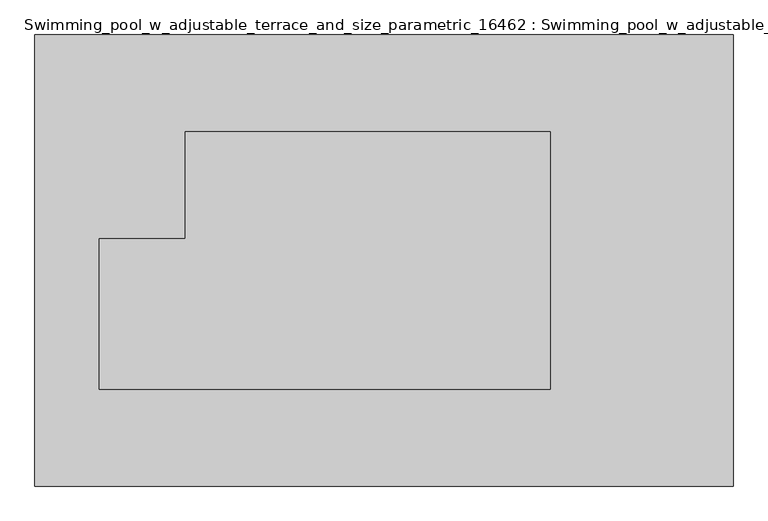
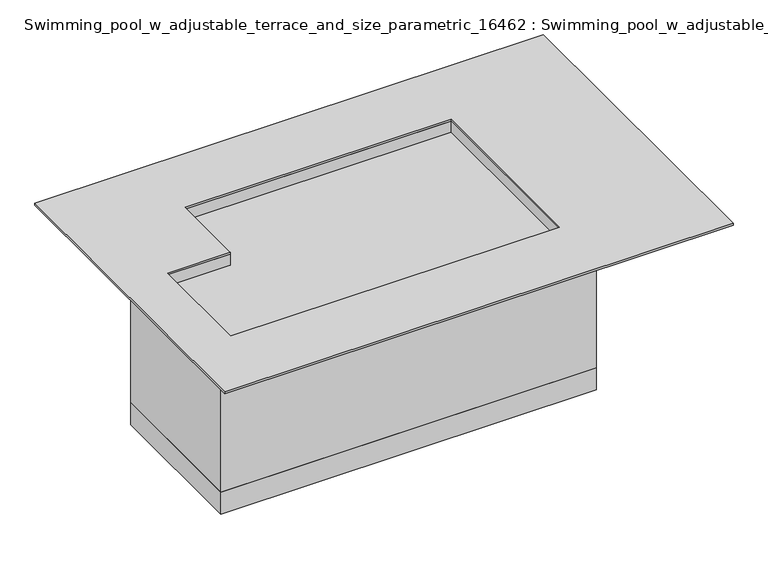
"""IFC4 building model written with IfcOpenShell, lengths in millimetres: furniture geometry, Swimming_pool_w_adjustable_terrace_and_size_parametric_16462 : Swimming_pool_w_adjustable_terrace_and_size_parametric_16462."""

from ifc_helpers import new_model, si_unit, frame, origin, origin_with_axes, place, context, project, spatial, polyline, outline, extrude, source, transform, mapped, element, save


def swimming_pool_w_adjustable_terrace_and_size_parametric_16462_e4165495(model_context):
    return source(origin(), model_context, "Body", "SweptSolid", [
        extrude(outline(polyline([(2400.0, 1500.0), (2400.0, -1500.0), (-2400.0, -1500.0), (-2400.0, 500.0), (-1600.0, 500.0), (-1600.0, 1500.0), (2400.0, 1500.0)]), holes=[polyline([(2100.0, 1200.0), (-1300.0, 1200.0), (-1300.0, 200.0), (-2100.0, 200.0), (-2100.0, -1200.0), (2100.0, -1200.0), (2100.0, 1200.0)])]), frame((0.0, 0.0, -1800.0), z_axis=(0.0, 0.0, 1.0), x_axis=(1.0, 0.0, 0.0)), (0.0, 0.0, 1.0), 1800.0),
        extrude(outline(polyline([(2400.0, 1500.0), (2400.0, -1500.0), (-2400.0, -1500.0), (-2400.0, 500.0), (-1600.0, 500.0), (-1600.0, 1500.0), (2400.0, 1500.0)])), frame((0.0, 0.0, -2100.0), z_axis=(0.0, 0.0, 1.0), x_axis=(1.0, 0.0, 0.0)), (0.0, 0.0, 1.0), 300.0),
        extrude(outline(polyline([(2100.0, 1200.0), (2100.0, -1200.0), (-2100.0, -1200.0), (-2100.0, 200.0), (-1300.0, 200.0), (-1300.0, 1200.0), (2100.0, 1200.0)])), frame((0.0, 0.0, -1800.0), z_axis=(0.0, 0.0, 1.0), x_axis=(1.0, 0.0, 0.0)), (0.0, 0.0, 1.0), 1650.0),
        extrude(outline(polyline([(3800.0, 2100.0), (3800.0, -2100.0), (-2700.0, -2100.0), (-2700.0, 2100.0), (3800.0, 2100.0)]), holes=[polyline([(2100.0, 1200.0), (-1300.0, 1200.0), (-1300.0, 200.0), (-2100.0, 200.0), (-2100.0, -1200.0), (2100.0, -1200.0), (2100.0, 1200.0)])]), origin_with_axes(), (0.0, 0.0, 1.0), 25.0),
    ])


if __name__ == "__main__":
    model = new_model("IFC4")
    model_context = context("Model", 3, world=origin())
    ifc_project = project(units=[si_unit("LENGTHUNIT", "METRE", prefix="MILLI")], contexts=[model_context])
    site = spatial("IfcSite", under=ifc_project)
    building = spatial("IfcBuilding", under=site)
    placement = place(None, origin())
    swimming_pool_w_adjustable_terrace_and_size_parametric_16462_shape = swimming_pool_w_adjustable_terrace_and_size_parametric_16462_e4165495(model_context)
    element("IfcFurniture", 1, ObjectType="Swimming_pool_w_adjustable_terrace_and_size_parametric_16462 : Swimming_pool_w_adjustable_terrace_and_size_parametric_16462", at=placement, inside=building, context=model_context, shape_type="MappedRepresentation", body=[
        mapped(swimming_pool_w_adjustable_terrace_and_size_parametric_16462_shape, transform((0.0, 0.0, 0.0), x_axis=(1.0, 0.0, 0.0), y_axis=(0.0, 1.0, 0.0), z_axis=(0.0, 0.0, 1.0))),
    ])
    save(model, "model.ifc")

# Revit data of these elements
# Type "Swimming_pool_w_adjustable_terrace_and_size_parametric_16462 : Swimming_pool_w_adjustable_terrace_and_size_parametric_16462"
#   Terrace thickness = 0' - 0.98425"
#   Terrace dimension back = 4' - 7.11811"
#   Terrace dimension side B = 1' - 11.62205"
#   Terrace dimemsion side A = 1' - 11.62205"
#   Terrace dimension front = 0' - 11.81102"
#   Water level/depth = 0' - 5.90551"
#   Length = 15' - 8.97638"
#   Width = 9' - 10.11024"
#   Depth pool = 5' - 10.86614"
#   Wall thickness = 0' - 11.81102"
#   Slab thickness = 0' - 11.81102"
#   Corner placement (on the left) = 3' - 3.37008"
#   Visibility water (yes/no) [instance default] = yes
#   Default Elevation = 0
